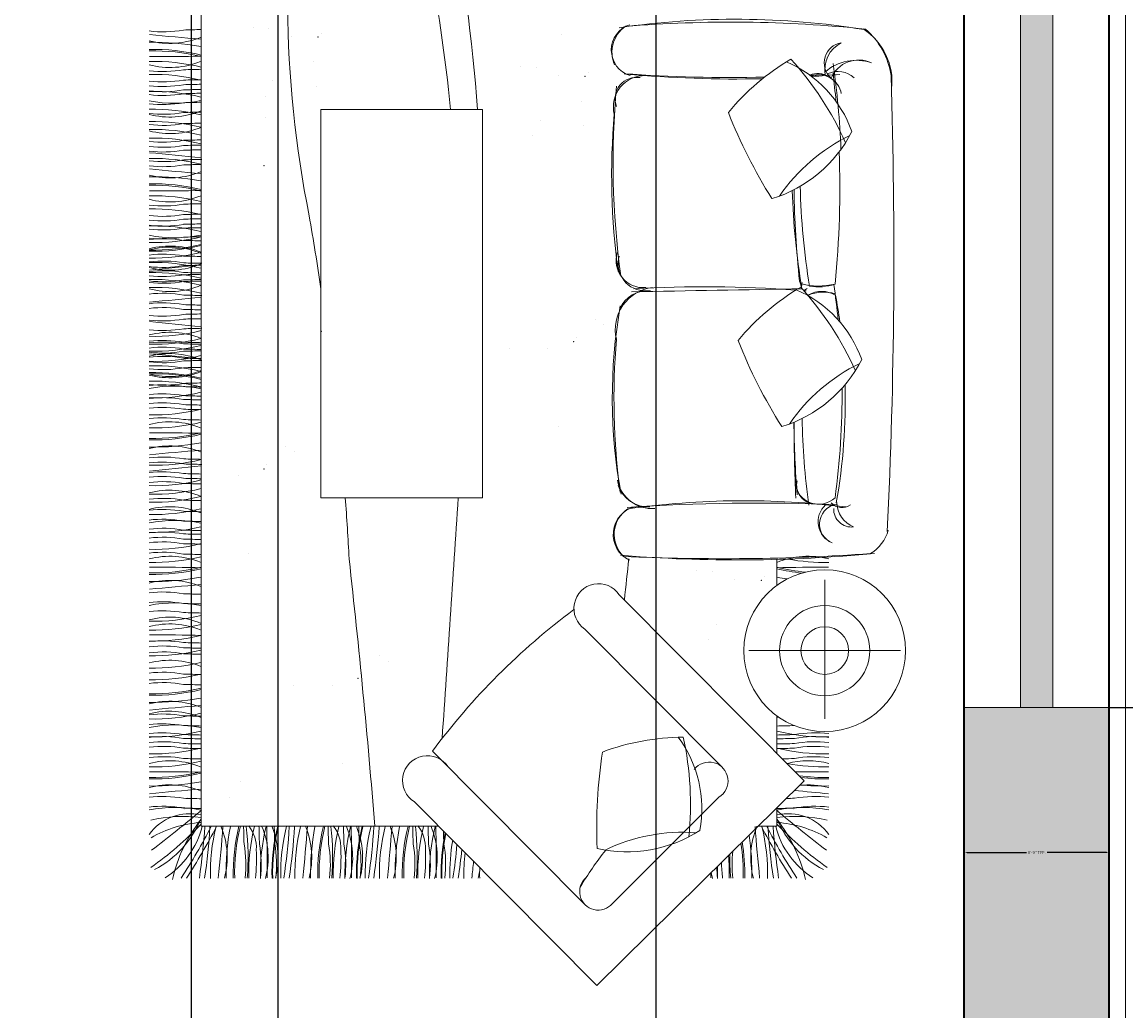
# Model space of a CAD drawing. Units: inches. Extents: x 311 to 815, y -527 to 136.
# Tile 11 of 21: x 655 to 723, y -464 to -403. Entities that reach past the tile are written whole.
import ezdxf

# ---------------------------------------------------------------- set-up
doc = ezdxf.new("R2010")
doc.units = ezdxf.units.IN
doc.header["$MEASUREMENT"] = 0
for name, color, linetype, lineweight in [('A-ANNO-DIMS', 1, 'Continuous', 18), ('A-FLOR-EDGE', 1, 'Continuous', 18), ('A-GLAZ-PATT', 5, 'Continuous', 13), ('A-WALL-PATT', 242, 'Continuous', 13), ('wall', 1, 'Continuous', 35), ('win', 5, 'Continuous', 18)]:
    doc.layers.add(name, color=color, linetype=linetype, lineweight=lineweight)
doc.layers.add('furniture', color=50, linetype='Continuous', lineweight=13, transparency=0.8)
doc.styles.get("Standard").update_dxf_attribs({"font": 'arial.ttf'})
doc.dimstyles.get("Standard").update_dxf_attribs({"dimtxt": 0.18, "dimasz": 0.18, "dimexe": 0.18, "dimexo": 0.0625, "dimgap": 0.09, "dimtad": 0, "dimtih": 1, "dimtoh": 1, "dimdec": 1, "dimzin": 0, "dimdsep": 46, "dimlunit": 4, "dimtxsty": 'Standard', "dimcen": 0.09, "dimadec": 0, "dimazin": 0, "dimtfac": 1, "dimtdec": 1, "dimtofl": 0, "dimtmove": 0, "dimatfit": 3, "dimfxl": 1, "dimtolj": 1, "dimtzin": 0, "dimarcsym": 0})

# ---------------------------------------------------------------- blocks, each defined once
blk = doc.blocks.new('WIN-60IN')
for p, q in [((9, 60), (0, 60)), ((3.5, 0), (3.5, 60)), ((5.5, 0), (5.5, 60)), ((9, 0), (0, 0))]:
    blk.add_line(p, q)
blk = doc.blocks.new('*D10')
at = {"layer": 'A-ANNO-DIMS', "color": 0, "lineweight": -2, "transparency": 16777216}
for p, q in [((722.385, -385.128), (731.503, -385.128)), ((731.323, -385.308), (731.323, -414.945)), ((731.323, -444.948), (731.323, -415.311)), ((722.385, -445.128), (731.503, -445.128))]:
    blk.add_line(p, q, dxfattribs=at)
at = {"layer": 'A-ANNO-DIMS', "color": 0, "transparency": 16777216}
for points in [[(731.293, -385.308), (731.353, -385.308), (731.323, -385.128)], [(731.293, -444.948), (731.353, -444.948), (731.323, -445.128)]]:
    blk.add_solid(points, dxfattribs=at)
at = {"layer": 'Defpoints', "color": 0, "transparency": 16777216}
for p in [(722.323, -385.128), (731.323, -385.128), (722.323, -445.128)]:
    blk.add_point(p, dxfattribs=at)
at = {"layer": 'A-ANNO-DIMS', "color": 0, "transparency": 16777216, "insert": (731.323, -415.128), "char_height": 0.18, "attachment_point": 5}
blk.add_mtext('\\A1;WINDOW 5\'-0" TYP.', dxfattribs=at)
blk = doc.blocks.new('*D11')
at = {"layer": 'A-ANNO-DIMS', "color": 0, "lineweight": -2, "transparency": 16777216}
for p, q in [((713.323, -445.19), (713.323, -454.308)), ((722.323, -445.19), (722.323, -454.308)), ((713.503, -454.128), (717.184, -454.128)), ((722.143, -454.128), (718.461, -454.128))]:
    blk.add_line(p, q, dxfattribs=at)
at = {"layer": 'A-ANNO-DIMS', "color": 0, "transparency": 16777216}
for points in [[(713.503, -454.098), (713.503, -454.158), (713.323, -454.128)], [(722.143, -454.098), (722.143, -454.158), (722.323, -454.128)]]:
    blk.add_solid(points, dxfattribs=at)
at = {"layer": 'Defpoints', "color": 0, "transparency": 16777216}
for p in [(713.323, -445.128), (722.323, -445.128), (722.323, -454.128)]:
    blk.add_point(p, dxfattribs=at)
at = {"layer": 'A-ANNO-DIMS', "color": 0, "transparency": 16777216, "insert": (717.823, -454.128), "char_height": 0.18, "attachment_point": 5}
blk.add_mtext('\\A1;0\'-9" TYP.', dxfattribs=at)
blk = doc.blocks.new('*D30')
at = {"layer": 'A-ANNO-DIMS', "color": 0, "lineweight": -2, "transparency": 16777216}
for p, q in [((722.385, -445.128), (754.853, -445.128)), ((754.673, -445.308), (754.673, -463.446)), ((754.673, -481.948), (754.673, -463.81)), ((722.385, -482.128), (754.853, -482.128))]:
    blk.add_line(p, q, dxfattribs=at)
at = {"layer": 'A-ANNO-DIMS', "color": 0, "transparency": 16777216}
for points in [[(754.643, -445.308), (754.703, -445.308), (754.673, -445.128)], [(754.643, -481.948), (754.703, -481.948), (754.673, -482.128)]]:
    blk.add_solid(points, dxfattribs=at)
at = {"layer": 'Defpoints', "color": 0, "transparency": 16777216}
for p in [(722.323, -445.128), (754.673, -445.128), (722.323, -482.128)]:
    blk.add_point(p, dxfattribs=at)
at = {"layer": 'A-ANNO-DIMS', "color": 0, "transparency": 16777216, "insert": (754.673, -463.628), "char_height": 0.18, "attachment_point": 5}
blk.add_mtext('\\A1;3\'-1"', dxfattribs=at)
blk = doc.blocks.new('*D31')
at = {"layer": 'A-ANNO-DIMS', "color": 0, "lineweight": -2, "transparency": 16777216}
for p, q in [((670.696, -191.608), (670.696, -526.658)), ((694.164, -191.608), (694.164, -526.658)), ((670.876, -526.478), (681.83, -526.478)), ((693.984, -526.478), (683.03, -526.478))]:
    blk.add_line(p, q, dxfattribs=at)
at = {"layer": 'A-ANNO-DIMS', "color": 0, "transparency": 16777216}
for points in [[(670.876, -526.448), (670.876, -526.508), (670.696, -526.478)], [(693.984, -526.448), (693.984, -526.508), (694.164, -526.478)]]:
    blk.add_solid(points, dxfattribs=at)
at = {"layer": 'Defpoints', "color": 0, "transparency": 16777216}
for p in [(670.696, -191.545), (694.164, -191.545), (694.164, -526.478)]:
    blk.add_point(p, dxfattribs=at)
at = {"layer": 'A-ANNO-DIMS', "color": 0, "transparency": 16777216, "insert": (682.43, -526.478), "char_height": 0.18, "attachment_point": 5}
blk.add_mtext('\\A1;1\'-11 1/2"', dxfattribs=at)
blk = doc.blocks.new('*D37')
at = {"layer": 'A-ANNO-DIMS', "color": 0, "lineweight": -2, "transparency": 16777216}
for p, q in [((633.323, -348.19), (633.323, -526.658)), ((665.323, -348.19), (665.323, -526.658)), ((633.503, -526.478), (648.992, -526.478)), ((665.143, -526.478), (649.654, -526.478))]:
    blk.add_line(p, q, dxfattribs=at)
at = {"layer": 'A-ANNO-DIMS', "color": 0, "transparency": 16777216}
for points in [[(633.503, -526.448), (633.503, -526.508), (633.323, -526.478)], [(665.143, -526.448), (665.143, -526.508), (665.323, -526.478)]]:
    blk.add_solid(points, dxfattribs=at)
at = {"layer": 'Defpoints', "color": 0, "transparency": 16777216}
for p in [(633.323, -348.128), (665.323, -348.128), (665.323, -526.478)]:
    blk.add_point(p, dxfattribs=at)
at = {"layer": 'A-ANNO-DIMS', "color": 0, "transparency": 16777216, "insert": (649.323, -526.478), "char_height": 0.18, "attachment_point": 5}
blk.add_mtext('\\A1;2\'-8"', dxfattribs=at)

msp = doc.modelspace()

# ---------------------------------------------------------------- hatches: boundary and pattern name
at = {"layer": 'A-GLAZ-PATT'}
h = msp.add_hatch(color=256, dxfattribs=at)
h.dxf.hatch_style = 1
h.paths.add_polyline_path([(415.823, -202.128), (413.823, -202.128), (413.823, -262.128), (415.823, -262.128)])
h.paths.add_polyline_path([(415.823, -390.84), (413.823, -390.84), (413.823, -450.84), (415.823, -450.84)])
h.paths.add_polyline_path([(415.823, -311.568), (413.823, -311.568), (413.823, -335.568), (415.823, -335.568)])
h.paths.add_polyline_path([(509.323, -476.628), (449.323, -476.628), (449.323, -478.628), (509.323, -478.628)])
h.paths.add_polyline_path([(606.823, -476.628), (582.823, -476.628), (582.823, -478.628), (606.823, -478.628)])
h.paths.add_polyline_path([(678.823, -476.628), (654.823, -476.628), (654.823, -478.628), (678.823, -478.628)])
h.paths.add_polyline_path([(718.823, -385.128), (716.823, -385.128), (716.823, -445.128), (718.823, -445.128)])
h.paths.add_polyline_path([(718.823, -262.628), (716.823, -262.628), (716.823, -322.628), (718.823, -322.628)])
h.paths.add_polyline_path([(718.823, -140.128), (716.823, -140.128), (716.823, -200.128), (718.823, -200.128)])
h.paths.add_polyline_path([(718.823, -18.128), (716.823, -18.128), (716.823, -42.128), (718.823, -42.128)])
h.paths.add_polyline_path([(686.823, 18.372), (626.823, 18.372), (626.823, 16.372), (686.823, 16.372)])
h.paths.add_polyline_path([(581.823, 18.372), (557.823, 18.372), (557.823, 16.372), (581.823, 16.372)])
h.paths.add_polyline_path([(509.323, 18.372), (449.323, 18.372), (449.323, 16.372), (509.323, 16.372)])
at = {"layer": 'A-WALL-PATT'}
h = msp.add_hatch(color=256, dxfattribs=at)
h.dxf.hatch_style = 1
h.paths.add_polyline_path([(557.823, 21.872), (509.323, 21.872), (509.323, 12.872), (539.323, 12.872), (539.323, -112.128), (548.323, -112.128), (548.323, -58.628), (557.823, -58.628), (557.823, -49.628), (548.323, -49.628), (548.323, 12.872), (557.823, 12.872)])
h.paths.add_polyline_path([(449.323, 21.872), (410.323, 21.872), (410.323, -15.128), (419.323, -15.128), (419.323, 12.872), (449.323, 12.872)])
h.paths.add_polyline_path([(626.823, 21.872), (581.823, 21.872), (581.823, 12.872), (591.323, 12.872), (591.323, -49.628), (581.823, -49.628), (581.823, -58.628), (591.323, -58.628), (591.323, -112.128), (600.323, -112.128), (600.323, 12.872), (626.823, 12.872)])
h.paths.add_polyline_path([(722.323, 21.872), (686.823, 21.872), (686.823, 12.872), (713.323, 12.872), (713.323, -18.128), (722.323, -18.128)])
h.paths.add_polyline_path([(722.323, -42.128), (713.323, -42.128), (713.323, -73.128), (722.323, -73.128)])
h.paths.add_polyline_path([(501.323, -103.128), (419.323, -103.128), (419.323, -75.128), (410.323, -75.128), (410.323, -126.628), (419.323, -126.628), (419.323, -112.128), (492.323, -112.128), (492.323, -143.128), (501.323, -143.128)])
h.paths.add_polyline_path([(548.323, -165.128), (419.323, -165.128), (419.323, -150.628), (410.323, -150.628), (410.323, -202.128), (419.323, -202.128), (419.323, -174.128), (548.323, -174.128)])
h.paths.add_polyline_path([(722.323, -103.128), (636.323, -103.128), (636.323, -112.128), (713.323, -112.128), (713.323, -140.128), (722.323, -140.128)])
h.paths.add_polyline_path([(548.323, -210.128), (539.323, -210.128), (539.323, -290.128), (419.323, -290.128), (419.323, -262.128), (410.323, -262.128), (410.323, -311.568), (419.323, -311.568), (419.323, -299.128), (469.323, -299.128), (469.323, -348.128), (443.323, -348.128), (443.323, -357.128), (478.323, -357.128), (478.323, -299.128), (548.323, -299.128)])
h.paths.add_polyline_path([(722.323, -200.128), (713.323, -200.128), (713.323, -228.128), (609.323, -228.128), (609.323, -237.128), (713.323, -237.128), (713.323, -262.628), (722.323, -262.628)])
h.paths.add_polyline_path([(722.323, -322.628), (713.323, -322.628), (713.323, -348.128), (633.323, -348.128), (633.323, -357.128), (713.323, -357.128), (713.323, -385.128), (722.323, -385.128)])
h.paths.add_polyline_path([(419.323, -335.568), (410.323, -335.568), (410.323, -390.84), (419.323, -390.84)])
h.paths.add_polyline_path([(419.323, -450.84), (410.323, -450.84), (410.323, -482.128), (449.323, -482.128), (449.323, -473.128), (419.323, -473.128)])
h.paths.add_polyline_path([(582.823, -473.128), (548.323, -473.128), (548.323, -348.128), (539.323, -348.128), (539.323, -473.128), (509.323, -473.128), (509.323, -482.128), (582.823, -482.128)])
h.paths.add_polyline_path([(722.323, -445.128), (713.323, -445.128), (713.323, -473.128), (678.823, -473.128), (678.823, -482.128), (722.323, -482.128)])

# ---------------------------------------------------------------- linework, layer by layer
at = {"layer": 'A-FLOR-EDGE'}
msp.add_line((723.323, -483.128), (723.323, 22.872), dxfattribs=at)
at = {"layer": 'furniture'}
for p, q in [((665.936, -452.501), (665.936, -388.632)), ((665.936, -398.727), (665.936, -452.501)), ((669.173, -402.89), (669.173, -402.89)), ((670.143, -402.965), (670.143, -402.965)), ((671.534, -403.459), (671.534, -403.459)), ((673.409, -403.275), (673.409, -403.275)), ((688.316, -403.329), (688.316, -403.329)), ((672.946, -405.051), (672.946, -405.051)), ((685.767, -405.34), (685.767, -405.34)), ((686.738, -405.415), (686.738, -405.415)), ((690.003, -405.725), (690.003, -405.725)), ((670.397, -406.214), (670.397, -406.214)), ((688.129, -405.909), (688.129, -405.909)), ((673.075, -406.567), (673.075, -406.567)), ((669.935, -407.168), (669.935, -407.168)), ((689.541, -407.501), (689.541, -407.501)), ((673.371, -408), (683.413, -408)), ((673.371, -432.102), (673.371, -408)), ((683.413, -408), (683.413, -432.102)), ((669.912, -408.488), (669.912, -408.488)), ((686.991, -408.665), (686.991, -408.665)), ((689.67, -409.017), (689.67, -409.017)), ((686.53, -409.618), (686.53, -409.618)), ((664.928, -416.035), (664.928, -416.035)), ((664.928, -416.106), (664.928, -416.106)), ((664.928, -418.285), (664.928, -418.285)), ((690.421, -421.011), (690.421, -421.011)), ((690.421, -421.011), (690.421, -421.011)), ((690.946, -421.359), (690.946, -421.359)), ((690.946, -421.359), (690.946, -421.359)), ((689.22, -422.136), (689.22, -422.136)), ((664.928, -422.848), (664.928, -422.848)), ((687.469, -422.829), (687.469, -422.829)), ((685.087, -422.864), (685.087, -422.864)), ((664.928, -425.027), (664.928, -425.027)), ((664.928, -425.098), (664.928, -425.098)), ((688.108, -427.669), (688.108, -427.669)), ((671.187, -428.913), (671.187, -428.913)), ((671.187, -428.913), (671.187, -428.913)), ((671.712, -429.261), (671.712, -429.261)), ((671.712, -429.261), (671.712, -429.261)), ((669.986, -430.038), (669.986, -430.038)), ((665.853, -430.766), (665.853, -430.766)), ((668.235, -430.73), (668.235, -430.73)), ((683.413, -432.102), (673.371, -432.102)), ((668.874, -435.571), (668.874, -435.571)), ((701.687, -435.93), (701.687, -437.547)), ((696.705, -436.628), (696.705, -436.628)), ((697.675, -436.702), (697.675, -436.702)), ((699.066, -437.197), (699.066, -437.197)), ((700.941, -437.012), (700.941, -437.012)), ((704.658, -441.595), (704.658, -437.2)), ((703.381, -449.674), (691.898, -438.125)), ((697.929, -439.952), (697.929, -439.952)), ((698.312, -448.858), (689.768, -440.255)), ((697.467, -440.905), (697.467, -440.905)), ((677.033, -441.918), (677.033, -441.918)), ((677.033, -441.918), (677.033, -441.918)), ((704.658, -441.595), (699.955, -441.595)), ((704.658, -441.595), (704.658, -445.828)), ((704.658, -441.595), (709.36, -441.595)), ((677.558, -442.266), (677.558, -442.266)), ((677.558, -442.266), (677.558, -442.266)), ((675.832, -443.043), (675.832, -443.043)), ((671.699, -443.771), (671.699, -443.771)), ((674.081, -443.735), (674.081, -443.735)), ((701.687, -445.643), (701.687, -447.971)), ((680.299, -447.842), (689.78, -457.369)), ((674.72, -448.576), (674.72, -448.576)), ((668.364, -449.733), (668.364, -449.733)), ((703.381, -449.674), (690.515, -462.379)), ((665.118, -450.713), (665.118, -450.713)), ((665.118, -450.713), (665.118, -450.713)), ((665.118, -450.713), (665.118, -450.713)), ((667.679, -450.695), (667.679, -450.695)), ((698.077, -450.697), (691.477, -457.296)), ((698.077, -450.697), (697.019, -451.755)), ((702.505, -450.713), (702.505, -450.713)), ((702.505, -450.713), (702.505, -450.713)), ((702.505, -450.713), (702.505, -450.713)), ((664.928, -451.486), (664.928, -451.486)), ((664.928, -451.486), (664.928, -451.486)), ((664.928, -451.486), (664.928, -451.486)), ((690.515, -462.379), (679.179, -450.979)), ((701.687, -451.347), (701.687, -452.501)), ((702.695, -451.486), (702.695, -451.486)), ((702.695, -451.486), (702.695, -451.486)), ((702.695, -451.486), (702.695, -451.486)), ((680.693, -452.501), (665.936, -452.501)), ((701.687, -452.501), (700.518, -452.501)), ((695.158, -453.615), (691.477, -457.296)), ((670.763, -454.219), (670.763, -454.219)), ((676.009, -454.219), (676.009, -454.219)), ((681.262, -454.219), (681.262, -454.219)), ((670.738, -454.523), (670.738, -454.523)), ((675.984, -454.523), (675.984, -454.523)), ((681.237, -454.523), (681.237, -454.523))]:
    msp.add_line(p, q, dxfattribs=at)
for radius in [5.021, 2.803, 1.481]:
    msp.add_circle((704.658, -441.595), radius, dxfattribs=at)
for centre, radius, start, end in [((741.561, -400.92), 70.258, 169.92753, 191.22459), ((587.613, -416.937), 94.235, 5.44209, 17.47988), ((537.566, -419.76), 146.015, 4.61959, 9.75131), ((693.064, -404.316), 1.657, 107.71573, 252.84284), ((693.448, -404.459), 2, 126.0678, 202.6723), ((699.135, -452.295), 49.897, 80.80787, 98.3514), ((698.81, -483.677), 81.099, 84.0627, 94.62528), ((663.574, -395.915), 7.265, 263.11705, 280.06509), ((664.003, -398.882), 5.018, 255.13868, 292.69016), ((677.166, -261.215), 142.863, 264.19829, 265.48538), ((667.404, -484.064), 81.037, 91.02248, 91.81091), ((704.912, -406.292), 3.923, 353.87925, 57.10928), ((704.032, -406.62), 4.8, 8.65495, 48.71038), ((662.987, -420.078), 16.251, 79.59608, 90.98046), ((663.005, -416.508), 12.239, 76.14265, 91.36693), ((705.887, -405.1), 1.263, 99.29162, 227.62886), ((706.582, -405.556), 1.925, 117.84326, 189.86837), ((663.004, -417.253), 12.239, 76.14265, 91.36693), ((663.005, -416.599), 12.239, 76.14265, 91.36693), ((664, -400.377), 5.018, 255.13868, 292.69016), ((663.458, -299.941), 104.775, 269.60659, 271.37204), ((709.882, -417.405), 14.512, 120.30685, 140.5663), ((699.365, -411.841), 7.4, 19.45006, 66.76991), ((688.059, -418.059), 19.597, 24.08153, 42.27682), ((706.614, -407.901), 2.952, 71.24727, 131.13483), ((706.769, -406.797), 1.868, 64.87152, 156.7247), ((663.581, -398.382), 7.265, 263.11705, 280.06509), ((667.411, -486.531), 81.037, 91.02248, 91.81091), ((705.48, -407.13), 1.491, 47.72028, 114.44608), ((655.363, -412.415), 50.34, 2.2017, 8.30671), ((663.579, -399.024), 7.265, 263.11705, 280.06509), ((663.002, -418.063), 12.239, 76.14265, 91.36693), ((667.41, -487.174), 81.037, 91.02248, 91.81091), ((693.462, -407.828), 1.929, 87.65794, 194.09744), ((692.978, -407.341), 1.336, 80.26169, 201.01149), ((698.759, -316.368), 89.651, 265.80271, 271.38032), ((699.078, -332.35), 73.76, 264.74224, 271.33354), ((704.211, -407.043), 1.273, 57.73663, 112.23873), ((698.759, -316.368), 89.651, 273.19084, 273.78915), ((704.289, -407.275), 1.421, 10.62162, 109.19299), ((699.078, -332.35), 73.76, 273.71005, 275.06529), ((644.917, -412.878), 60.679, 5.08707, 6.74912), ((349.903, -417.097), 359.048, 357.2697, 1.7875), ((663.577, -399.868), 7.265, 263.11705, 280.06509), ((663.578, -399.633), 7.265, 263.11705, 280.06509), ((662.999, -419.116), 12.239, 76.14265, 91.36693), ((663.578, -399.312), 7.265, 263.11705, 280.06509), ((667.407, -488.017), 81.037, 91.02248, 91.81091), ((667.408, -487.782), 81.037, 91.02248, 91.81091), ((667.409, -487.461), 81.037, 91.02248, 91.81091), ((743.964, -411.292), 52.447, 174.82447, 187.71479), ((663.575, -400.428), 7.265, 263.11705, 280.06509), ((664.295, -399.481), 8.138, 258.75453, 281.58879), ((667.406, -488.577), 81.037, 91.02248, 91.81091), ((663.574, -401.035), 7.265, 263.11705, 280.06509), ((662.996, -420.226), 12.239, 76.14265, 91.36693), ((663.992, -403.454), 5.018, 255.13868, 292.69016), ((667.404, -489.184), 81.037, 91.02248, 91.81091), ((735.84, -412.109), 44.413, 175.07811, 187.69498), ((727.594, -396.89), 31.049, 201.33709, 212.41765), ((662.997, -420.987), 12.239, 76.14265, 91.36693), ((663.584, -401.724), 7.265, 263.11705, 280.06509), ((664.005, -404.48), 5.018, 255.13868, 292.69016), ((667.415, -489.874), 81.037, 91.02248, 91.81091), ((663.007, -422.016), 12.239, 76.14265, 91.36693), ((663.008, -421.481), 12.239, 76.14265, 91.36693), ((698.958, -405.605), 8.293, 287.0126, 332.9429), ((711.121, -419.709), 11.224, 115.90051, 145.65125), ((663.584, -403.084), 7.265, 263.11705, 280.06509), ((663.585, -402.763), 7.265, 263.11705, 280.06509), ((667.405, -491.527), 81.037, 91.02248, 91.81091), ((667.415, -491.233), 81.037, 91.02248, 91.81091), ((667.415, -490.912), 81.037, 91.02248, 91.81091), ((663.574, -403.377), 7.265, 263.11705, 280.06509), ((663.01, -423.28), 12.239, 76.14265, 91.36693), ((663.592, -403.975), 7.265, 263.11705, 280.06509), ((637.626, -681.199), 271.677, 84.01654, 84.69917), ((667.422, -492.124), 81.037, 91.02248, 91.81091), ((644.917, -412.878), 60.679, 354.36393, 2.12187), ((664.003, -407.228), 5.018, 255.13868, 292.69016), ((663.587, -404.288), 7.265, 263.11705, 280.06509), ((677.166, -269.561), 142.863, 264.19829, 265.48538), ((667.418, -492.437), 81.037, 91.02248, 91.81091), ((662.987, -428.423), 16.251, 79.59608, 90.98046), ((663.005, -424.854), 12.239, 76.14265, 91.36693), ((663.005, -424.945), 12.239, 76.14265, 91.36693), ((663.458, -308.286), 104.775, 269.60659, 271.37204), ((747.074, -411.756), 44.447, 181.64583, 189.52678), ((758.639, -412.494), 55.884, 180.49489, 186.32914), ((744.759, -412.035), 41.624, 181.00607, 189.60009), ((663.581, -406.728), 7.265, 263.11705, 280.06509), ((663.004, -425.599), 12.239, 76.14265, 91.36693), ((664, -408.723), 5.018, 255.13868, 292.69016), ((667.411, -494.877), 81.037, 91.02248, 91.81091), ((663.579, -407.37), 7.265, 263.11705, 280.06509), ((663.002, -426.409), 12.239, 76.14265, 91.36693), ((667.41, -495.519), 81.037, 91.02248, 91.81091), ((538.237, -438.403), 136.502, 8.11901, 10.04424), ((663.578, -407.978), 7.265, 263.11705, 280.06509), ((662.999, -427.461), 12.239, 76.14265, 91.36693), ((663.578, -407.657), 7.265, 263.11705, 280.06509), ((667.408, -496.127), 81.037, 91.02248, 91.81091), ((667.409, -495.807), 81.037, 91.02248, 91.81091), ((663.575, -408.774), 7.265, 263.11705, 280.06509), ((663.577, -408.214), 7.265, 263.11705, 280.06509), ((664.295, -407.827), 8.138, 258.75453, 281.58879), ((663.007, -404.029), 12.239, 268.63307, 283.85735), ((667.406, -496.923), 81.037, 91.02248, 91.81091), ((667.407, -496.363), 81.037, 91.02248, 91.81091), ((663.585, -423.282), 7.265, 79.93491, 96.88295), ((663.008, -404.493), 12.239, 268.63307, 283.85735), ((663.008, -404.564), 12.239, 268.63307, 283.85735), ((664.005, -421.494), 5.018, 67.30984, 104.86132), ((664.005, -421.565), 5.018, 67.30984, 104.86132), ((667.415, -335.132), 81.037, 268.18909, 268.97752), ((662.997, -404.987), 12.239, 268.63307, 283.85735), ((663.584, -424.25), 7.265, 79.93491, 96.88295), ((667.415, -336.101), 81.037, 268.18909, 268.97752), ((693.39, -417.372), 1.691, 162.93165, 275.10915), ((693.511, -417.581), 1.676, 163.4437, 271.82282), ((663.574, -410.542), 7.265, 263.11705, 280.06509), ((662.996, -429.733), 12.239, 76.14265, 91.36693), ((663.574, -425.274), 7.265, 79.93491, 96.88295), ((663.992, -412.961), 5.018, 255.13868, 292.69016), ((663.592, -424.676), 7.265, 79.93491, 96.88295), ((637.626, -147.452), 271.677, 275.30083, 275.98346), ((667.404, -498.691), 81.037, 91.02248, 91.81091), ((667.422, -336.527), 81.037, 268.18909, 268.97752), ((662.997, -430.791), 12.239, 76.14265, 91.36693), ((663.584, -411.43), 7.265, 263.11705, 280.06509), ((663.585, -411.109), 7.265, 263.11705, 280.06509), ((663.584, -411.529), 7.265, 263.11705, 280.06509), ((663.007, -430.361), 12.239, 76.14265, 91.36693), ((667.405, -337.124), 81.037, 268.18909, 268.97752), ((667.415, -499.579), 81.037, 91.02248, 91.81091), ((667.415, -499.678), 81.037, 91.02248, 91.81091), ((667.415, -499.258), 81.037, 91.02248, 91.81091), ((686.135, -423.99), 17.781, 15.96247, 17.46375), ((789.397, -427.959), 86.636, 173.88721, 174.12153), ((663.008, -431.286), 12.239, 76.14265, 91.36693), ((664.005, -414.285), 5.018, 255.13868, 292.69016), ((663.592, -426.673), 7.265, 79.93491, 96.88295), ((694.273, -421.657), 2.617, 96.58671, 193.45107), ((693.668, -421.168), 1.911, 84.92344, 155.63742), ((-15074.083, 884137.718), 884697.543, 271.021158169, 271.0218453), ((697.245, -496.583), 77.577, 85.84252, 93.2873), ((710.49, -431.56), 14.512, 120.30685, 140.5663), ((699.974, -425.996), 7.4, 19.45006, 66.76991), ((704.285, -414.819), 4.145, 254.04794, 284.20605), ((688.668, -432.214), 19.597, 24.08153, 42.27682), ((697.245, -496.583), 77.577, 85.36553, 85.4784), ((704.071, -420.036), 1.053, 119.13127, 132.01414), ((704.594, -421.806), 2.471, 73.31083, 112.61636), ((704.471, -420.974), 1.679, 59.83188, 119.46797), ((704.219, -415.607), 3.407, 261.53624, 288.34934), ((659.2, -425.759), 46.534, 5.77953, 8.52202), ((663.574, -427.271), 7.265, 79.93491, 96.88295), ((637.626, -149.449), 271.677, 275.30083, 275.98346), ((667.405, -339.121), 81.037, 268.18909, 268.97752), ((667.422, -338.524), 81.037, 268.18909, 268.97752), ((754.132, -425.971), 50.898, 172.72451, 172.77255), ((669.76, -426.096), 36.171, 7.80299, 10.45572), ((663.584, -427.564), 7.265, 79.93491, 96.88295), ((663.584, -413.569), 7.265, 263.11705, 280.06509), ((667.415, -339.415), 81.037, 268.18909, 268.97752), ((667.415, -501.718), 81.037, 91.02248, 91.81091), ((724.548, -425.909), 33.08, 170.0543, 190.4167), ((663.574, -413.863), 7.265, 263.11705, 280.06509), ((637.626, -691.684), 271.677, 84.01654, 84.69917), ((667.405, -502.012), 81.037, 91.02248, 91.81091), ((663.008, -409.848), 12.239, 268.63307, 283.85735), ((664.005, -426.849), 5.018, 67.30984, 104.86132), ((663.592, -414.46), 7.265, 263.11705, 280.06509), ((667.422, -502.609), 81.037, 91.02248, 91.81091), ((662.997, -410.342), 12.239, 268.63307, 283.85735), ((663.584, -429.703), 7.265, 79.93491, 96.88295), ((663.584, -429.604), 7.265, 79.93491, 96.88295), ((663.585, -430.024), 7.265, 79.93491, 96.88295), ((663.007, -410.772), 12.239, 268.63307, 283.85735), ((667.415, -341.455), 81.037, 268.18909, 268.97752), ((667.415, -341.554), 81.037, 268.18909, 268.97752), ((735.74, -425.956), 44.167, 175.20718, 187.55097), ((728.203, -411.045), 31.049, 201.33709, 212.41765), ((663.574, -430.591), 7.265, 79.93491, 96.88295), ((663.574, -415.86), 7.265, 263.11705, 280.06509), ((662.996, -411.4), 12.239, 268.63307, 283.85735), ((663.992, -428.172), 5.018, 67.30984, 104.86132), ((637.626, -693.681), 271.677, 84.01654, 84.69917), ((667.404, -342.442), 81.037, 268.18909, 268.97752), ((667.405, -504.009), 81.037, 91.02248, 91.81091), ((667.415, -341.875), 81.037, 268.18909, 268.97752), ((699.566, -419.76), 8.293, 287.0126, 332.9429), ((662.997, -436.146), 12.239, 76.14265, 91.36693), ((663.584, -416.883), 7.265, 263.11705, 280.06509), ((664.005, -419.568), 5.018, 255.13868, 292.69016), ((663.592, -416.457), 7.265, 263.11705, 280.06509), ((667.415, -505.033), 81.037, 91.02248, 91.81091), ((667.422, -504.606), 81.037, 91.02248, 91.81091), ((711.73, -433.863), 11.224, 115.90051, 145.65125), ((663.007, -437.104), 12.239, 76.14265, 91.36693), ((663.008, -436.569), 12.239, 76.14265, 91.36693), ((663.008, -436.64), 12.239, 76.14265, 91.36693), ((664.005, -419.639), 5.018, 255.13868, 292.69016), ((663.575, -432.359), 7.265, 79.93491, 96.88295), ((664.295, -433.306), 8.138, 78.41121, 101.24547), ((662.999, -413.672), 12.239, 268.63307, 283.85735), ((663.585, -417.852), 7.265, 263.11705, 280.06509), ((667.406, -344.21), 81.037, 268.18909, 268.97752), ((667.415, -506.001), 81.037, 91.02248, 91.81091), ((659.2, -425.759), 46.534, 352.15508, 0.55852), ((669.76, -426.096), 36.171, 349.94664, 1.59031), ((663.577, -432.919), 7.265, 79.93491, 96.88295), ((663.578, -433.155), 7.265, 79.93491, 96.88295), ((663.578, -433.476), 7.265, 79.93491, 96.88295), ((667.407, -344.77), 81.037, 268.18909, 268.97752), ((667.408, -345.006), 81.037, 268.18909, 268.97752), ((663.579, -433.763), 7.265, 79.93491, 96.88295), ((663.002, -414.725), 12.239, 268.63307, 283.85735), ((667.409, -345.327), 81.037, 268.18909, 268.97752), ((667.41, -345.614), 81.037, 268.18909, 268.97752), ((663.581, -434.405), 7.265, 79.93491, 96.88295), ((663.004, -415.534), 12.239, 268.63307, 283.85735), ((664, -432.41), 5.018, 67.30984, 104.86132), ((667.411, -346.256), 81.037, 268.18909, 268.97752), ((772.401, -426.514), 69.666, 180.7456, 184.45597), ((789.397, -427.959), 86.636, 179.63856, 182.76525), ((754.132, -425.971), 50.898, 181.37312, 187.44721), ((663.005, -416.188), 12.239, 268.63307, 283.85735), ((663.005, -416.279), 12.239, 268.63307, 283.85735), ((663.458, -532.847), 104.775, 88.62796, 90.39341), ((662.987, -412.71), 16.251, 269.01954, 280.40392), ((664.003, -433.905), 5.018, 67.30984, 104.86132), ((663.587, -436.845), 7.265, 79.93491, 96.88295), ((677.166, -571.573), 142.863, 94.51462, 95.80171), ((667.418, -348.696), 81.037, 268.18909, 268.97752), ((663.01, -417.853), 12.239, 268.63307, 283.85735), ((663.592, -437.158), 7.265, 79.93491, 96.88295), ((637.626, -159.934), 271.677, 275.30083, 275.98346), ((667.422, -349.009), 81.037, 268.18909, 268.97752), ((663.574, -437.756), 7.265, 79.93491, 96.88295), ((663.584, -438.049), 7.265, 79.93491, 96.88295), ((663.007, -419.117), 12.239, 268.63307, 283.85735), ((667.405, -349.607), 81.037, 268.18909, 268.97752), ((667.415, -349.9), 81.037, 268.18909, 268.97752), ((693.923, -430.603), 2.173, 190.97559, 274.97468), ((704.085, -431.313), 1.171, 167.62255, 260.30943), ((663.585, -438.37), 7.265, 79.93491, 96.88295), ((663.008, -419.652), 12.239, 268.63307, 283.85735), ((664.005, -436.653), 5.018, 67.30984, 104.86132), ((667.415, -350.221), 81.037, 268.18909, 268.97752), ((693.721, -430.663), 2.012, 199.82281, 272.49854), ((704.289, -431.031), 1.478, 186.1174, 313.1189), ((662.997, -420.146), 12.239, 268.63307, 283.85735), ((663.584, -439.409), 7.265, 79.93491, 96.88295), ((667.415, -351.26), 81.037, 268.18909, 268.97752), ((546.734, -442.144), 128.547, 2.78771, 4.48071), ((-2183.497, -248.346), 2871.284, 356.03178, 356.330686), ((700.403, -548.527), 116.093, 87.50734, 93.9592), ((699.641, -484.084), 51.795, 82.98362, 97.98903), ((705.734, -431.758), 0.952, 224.39377, 303.58565), ((707.087, -432.358), 1.684, 181.18396, 247.82163), ((663.574, -440.098), 7.265, 79.93491, 96.88295), ((662.996, -420.907), 12.239, 268.63307, 283.85735), ((663.992, -437.679), 5.018, 67.30984, 104.86132), ((667.404, -351.949), 81.037, 268.18909, 268.97752), ((693.303, -434.381), 1.776, 104.63788, 244.30948), ((693.474, -434.379), 1.893, 123.04105, 226.06525), ((705.655, -433.596), 1.413, 132.31343, 247.61024), ((705.597, -433.738), 1.26, 104.78136, 247.59217), ((706.324, -432.812), 1.112, 178.0108, 276.55846), ((663.575, -440.705), 7.265, 79.93491, 96.88295), ((664.295, -441.652), 8.138, 78.41121, 101.24547), ((667.406, -352.556), 81.037, 268.18909, 268.97752), ((663.577, -441.265), 7.265, 79.93491, 96.88295), ((662.999, -422.017), 12.239, 268.63307, 283.85735), ((663.578, -441.501), 7.265, 79.93491, 96.88295), ((667.407, -353.116), 81.037, 268.18909, 268.97752), ((667.408, -353.351), 81.037, 268.18909, 268.97752), ((706.165, -433.422), 2.536, 301.88171, 343.96721), ((663.578, -441.821), 7.265, 79.93491, 96.88295), ((663.579, -442.109), 7.265, 79.93491, 96.88295), ((663.002, -423.07), 12.239, 268.63307, 283.85735), ((667.409, -353.672), 81.037, 268.18909, 268.97752), ((667.41, -353.96), 81.037, 268.18909, 268.97752), ((663.581, -442.751), 7.265, 79.93491, 96.88295), ((663.004, -423.88), 12.239, 268.63307, 283.85735), ((664, -440.756), 5.018, 67.30984, 104.86132), ((667.411, -354.602), 81.037, 268.18909, 268.97752), ((699.186, -345.407), 90.558, 265.43246, 275.43098), ((698.389, -302.976), 132.912, 267.31429, 273.93296), ((703.623, -440.756), 5.018, 75.13868, 112.69016), ((663.005, -424.534), 12.239, 268.63307, 283.85735), ((663.005, -424.625), 12.239, 268.63307, 283.85735), ((663.458, -541.192), 104.775, 88.62796, 90.39341), ((85.648, -501.084), 593.075, 4.698728, 6.310761), ((1281.976, -501.084), 593.075, 173.689239, 173.937357), ((704.166, -541.192), 104.775, 89.60659, 91.37204), ((704.619, -424.534), 12.239, 256.14265, 264.58544), ((704.619, -424.625), 12.239, 256.14265, 263.44666), ((704.62, -423.88), 12.239, 259.37308, 271.36693), ((662.987, -421.055), 16.251, 269.01954, 280.40392), ((664.003, -442.251), 5.018, 67.30984, 104.86132), ((704.637, -421.055), 16.251, 259.59608, 261.86196), ((677.166, -579.918), 142.863, 94.51462, 95.80171), ((690.619, -438.976), 1.536, 33.6335, 236.3665), ((663.574, -445.218), 7.265, 79.93491, 96.88295), ((663.575, -445.825), 7.265, 79.93491, 96.88295), ((667.404, -357.069), 81.037, 268.18909, 268.97752), ((663.577, -446.385), 7.265, 79.93491, 96.88295), ((664.295, -446.772), 8.138, 78.41121, 101.24547), ((667.406, -357.676), 81.037, 268.18909, 268.97752), ((667.407, -358.236), 81.037, 268.18909, 268.97752), ((714.586, -473.31), 42.711, 126.66127, 143.39506), ((663.004, -428.08), 12.239, 268.63307, 283.85735), ((664, -444.956), 5.018, 67.30984, 104.86132), ((663.008, -427.533), 12.239, 268.63307, 283.85735), ((664.005, -444.534), 5.018, 67.30984, 104.86132), ((662.999, -428.766), 12.239, 268.63307, 283.85735), ((663.458, -545.392), 104.775, 88.62796, 90.39341), ((663.578, -448.249), 7.265, 79.93491, 96.88295), ((663.578, -448.57), 7.265, 79.93491, 96.88295), ((667.408, -360.1), 81.037, 268.18909, 268.97752), ((662.997, -429.679), 12.239, 268.63307, 283.85735), ((663.584, -448.942), 7.265, 79.93491, 96.88295), ((667.409, -360.421), 81.037, 268.18909, 268.97752), ((667.415, -360.793), 81.037, 268.18909, 268.97752), ((662.996, -430.44), 12.239, 268.63307, 283.85735), ((663.992, -447.212), 5.018, 67.30984, 104.86132), ((663.579, -450.202), 7.265, 79.93491, 96.88295), ((663.002, -431.164), 12.239, 268.63307, 283.85735), ((667.41, -362.053), 81.037, 268.18909, 268.97752), ((663.581, -450.844), 7.265, 79.93491, 96.88295), ((663.005, -432.037), 12.239, 268.63307, 283.85735), ((663.005, -432.129), 12.239, 268.63307, 283.85735), ((667.411, -362.695), 81.037, 268.18909, 268.97752), ((662.987, -428.559), 16.251, 269.01954, 280.40392), ((664.003, -449.755), 5.018, 67.30984, 104.86132), ((663.992, -450.374), 5.018, 67.30984, 104.86132), ((677.166, -587.422), 142.863, 94.51462, 95.80171), ((663.574, -452.793), 7.265, 79.93491, 96.88295), ((662.996, -433.602), 12.239, 268.63307, 283.85735), ((663.575, -453.4), 7.265, 79.93491, 96.88295), ((667.404, -364.644), 81.037, 268.18909, 268.97752), ((700.219, -364.644), 81.037, 271.02248, 271.06056), ((703.631, -450.374), 5.018, 111.65199, 112.69016), ((663.577, -453.96), 7.265, 79.93491, 96.88295), ((664.295, -454.347), 8.138, 78.41121, 101.24547), ((662.999, -434.712), 12.239, 268.63307, 283.85735), ((667.406, -365.251), 81.037, 268.18909, 268.97752), ((667.407, -365.811), 81.037, 268.18909, 268.97752), ((700.216, -365.811), 81.037, 271.02248, 271.81091), ((700.218, -365.251), 81.037, 271.02248, 271.81091), ((704.625, -434.712), 12.239, 256.14265, 271.36693), ((704.047, -453.96), 7.265, 83.11705, 100.06509), ((663.578, -454.195), 7.265, 79.93491, 96.88295), ((663.578, -454.516), 7.265, 79.93491, 96.88295), ((667.408, -366.046), 81.037, 268.18909, 268.97752), ((667.409, -366.367), 81.037, 268.18909, 268.97752), ((695.953, -461.478), 14.512, 90.30685, 110.5663), ((689.627, -451.402), 7.4, 349.45006, 36.76991), ((676.727, -451.134), 19.597, 354.08153, 12.27682), ((700.215, -366.367), 81.037, 271.02248, 271.81091), ((700.216, -366.046), 81.037, 271.02248, 271.81091), ((704.046, -454.195), 7.265, 83.11705, 100.06509), ((704.045, -454.516), 7.265, 83.11705, 100.06509), ((663.579, -454.804), 7.265, 79.93491, 96.88295), ((663.002, -435.765), 12.239, 268.63307, 283.85735), ((663.581, -455.446), 7.265, 79.93491, 96.88295), ((667.41, -366.655), 81.037, 268.18909, 268.97752), ((679.986, -449.662), 1.544, 33.09238, 238.53066), ((721.55, -452.568), 31.049, 171.33709, 182.41765), ((700.214, -366.655), 81.037, 271.02248, 271.81091), ((704.622, -435.765), 12.239, 256.14265, 271.36693), ((704.043, -455.446), 7.265, 83.11705, 100.06509), ((704.044, -454.804), 7.265, 83.11705, 100.06509), ((663.004, -436.575), 12.239, 268.63307, 283.85735), ((664, -453.451), 5.018, 67.30984, 104.86132), ((667.411, -367.297), 81.037, 268.18909, 268.97752), ((697.482, -449.686), 1.172, 300.48188, 142.32523), ((700.212, -367.297), 81.037, 271.2964, 271.81091), ((703.623, -453.451), 5.018, 75.13868, 104.83406), ((704.62, -436.575), 12.239, 259.25336, 271.36693), ((663.005, -437.229), 12.239, 268.63307, 283.85735), ((663.005, -437.32), 12.239, 268.63307, 283.85735), ((663.458, -553.887), 104.775, 88.62796, 90.39341), ((704.166, -553.887), 104.775, 89.60659, 90.73035), ((704.619, -437.229), 12.239, 262.7707, 271.36693), ((704.619, -437.32), 12.239, 263.2584, 271.36693), ((662.987, -433.75), 16.251, 269.01954, 280.40392), ((664.003, -454.946), 5.018, 67.30984, 104.86132), ((677.166, -592.613), 142.863, 94.51462, 95.80171), ((703.621, -454.946), 5.018, 75.13868, 96.00411), ((704.637, -433.75), 16.251, 264.64881, 270.98046), ((663.574, -457.913), 7.265, 79.93491, 96.88295), ((667.404, -369.764), 81.037, 268.18909, 268.97752), ((700.219, -369.764), 81.037, 271.46162, 271.81091), ((690.457, -592.613), 142.863, 84.19829, 85.05746), ((704.05, -457.913), 7.265, 83.11705, 100.06509), ((663.575, -458.52), 7.265, 79.93491, 96.88295), ((664.295, -459.467), 8.138, 78.41121, 101.24547), ((602.458, -375.386), 99.132, 307.54408, 309.84318), ((667.406, -370.371), 81.037, 268.18909, 268.97752), ((765.166, -375.386), 99.132, 230.15682, 232.45592), ((700.218, -370.371), 81.037, 271.02248, 271.81091), ((703.329, -459.467), 8.138, 78.75453, 101.58879), ((704.048, -458.52), 7.265, 83.11705, 100.06509), ((665.244, -454.843), 3.126, 77.19461, 144.09429), ((664.838, -460.71), 8.827, 82.85092, 103.27854), ((666.483, -459.572), 7.336, 94.27565, 119.86497), ((660.203, -449.686), 6.189, 297.30329, 337.88189), ((673.427, -457.935), 9.516, 141.9231, 167.04771), ((702.38, -454.843), 3.126, 35.90571, 102.80539), ((702.786, -460.71), 8.827, 76.72146, 97.14908), ((707.421, -449.686), 6.189, 202.11811, 242.69671), ((694.196, -457.935), 9.516, 12.95229, 38.0769), ((701.14, -459.572), 7.336, 60.13503, 85.72435), ((650.334, -437.447), 21.587, 305.31527, 316.284), ((660.88, -451.227), 5.282, 302.27123, 346.00651), ((634.552, -436.002), 36.02, 326.82194, 332.73315), ((634.877, -436.01), 36.02, 326.82194, 332.73315), ((631.241, -450.469), 34.984, 351.37714, 356.63558), ((631.566, -450.477), 34.984, 351.37714, 356.63558), ((678.75, -455.439), 12.239, 166.14265, 181.36693), ((524.875, -441.271), 142.863, 354.19829, 355.48538), ((662.542, -454.435), 5.018, 345.13868, 22.69016), ((683.738, -455.451), 16.251, 169.59608, 180.98046), ((680.168, -455.433), 12.239, 166.14265, 181.36693), ((680.259, -455.433), 12.239, 166.14265, 181.36693), ((749.601, -451.026), 81.037, 181.02248, 181.81091), ((652.323, -454.431), 16.533, 355.49364, 6.62982), ((681.133, -455.436), 12.239, 166.14265, 181.36693), ((667.182, -453.832), 2.188, 356.82563, 38.34356), ((750.556, -451.03), 81.037, 181.02248, 181.81091), ((681.857, -455.442), 12.239, 166.14265, 181.36693), ((665.085, -454.445), 5.018, 345.13868, 22.69016), ((565.264, -454.98), 104.775, 359.60659, 1.37204), ((665.7, -454.437), 5.018, 345.13868, 22.69016), ((682.576, -455.434), 12.239, 166.14265, 181.36693), ((682.617, -455.44), 12.239, 166.14265, 181.36693), ((751.504, -451.023), 81.037, 181.02248, 181.81091), ((683.123, -455.429), 12.239, 166.14265, 181.36693), ((636.487, -450.469), 34.984, 351.37714, 356.63558), ((636.813, -450.477), 34.984, 351.37714, 356.63558), ((683.997, -455.439), 12.239, 166.14265, 181.36693), ((530.121, -441.271), 142.863, 354.19829, 355.48538), ((667.789, -454.435), 5.018, 345.13868, 22.69016), ((688.984, -455.451), 16.251, 169.59608, 180.98046), ((685.415, -455.433), 12.239, 166.14265, 181.36693), ((685.506, -455.433), 12.239, 166.14265, 181.36693), ((754.848, -451.026), 81.037, 181.02248, 181.81091), ((657.57, -454.431), 16.533, 355.49364, 6.62982), ((686.379, -455.436), 12.239, 166.14265, 181.36693), ((672.428, -453.832), 2.188, 356.82563, 38.34356), ((755.803, -451.03), 81.037, 181.02248, 181.81091), ((687.104, -455.442), 12.239, 166.14265, 181.36693), ((670.332, -454.445), 5.018, 345.13868, 22.69016), ((570.51, -454.98), 104.775, 359.60659, 1.37204), ((670.947, -454.437), 5.018, 345.13868, 22.69016), ((687.823, -455.434), 12.239, 166.14265, 181.36693), ((687.864, -455.44), 12.239, 166.14265, 181.36693), ((756.751, -451.023), 81.037, 181.02248, 181.81091), ((688.37, -455.429), 12.239, 166.14265, 181.36693), ((641.74, -450.469), 34.984, 351.37714, 356.63558), ((642.065, -450.477), 34.984, 351.37714, 356.63558), ((689.249, -455.439), 12.239, 166.14265, 181.36693), ((535.374, -441.271), 142.863, 354.19829, 355.48538), ((673.041, -454.435), 5.018, 345.13868, 22.69016), ((694.236, -455.451), 16.251, 169.59608, 180.98046), ((690.667, -455.433), 12.239, 166.14265, 181.36693), ((690.758, -455.433), 12.239, 166.14265, 181.36693), ((760.1, -451.026), 81.037, 181.02248, 181.81091), ((662.822, -454.431), 16.533, 355.49364, 6.62982), ((691.632, -455.436), 12.239, 166.14265, 181.36693), ((677.681, -453.832), 2.188, 356.82563, 38.34356), ((761.055, -451.03), 81.037, 181.02248, 181.81091), ((692.356, -455.442), 12.239, 166.14265, 181.36693), ((675.584, -454.445), 5.018, 345.13868, 22.69016), ((575.763, -454.98), 104.775, 359.60659, 1.37204), ((693.075, -455.434), 12.239, 168.09925, 181.36693), ((693.116, -455.44), 12.239, 168.23618, 181.36693), ((762.003, -451.023), 81.037, 181.25348, 181.81091), ((692.393, -445.797), 8.293, 257.0126, 302.9429), ((695.875, -464.093), 11.224, 85.90051, 115.65125), ((705.081, -454.435), 5.018, 157.30984, 194.86132), ((842.749, -441.271), 142.863, 184.51462, 185.80171), ((732.746, -436.01), 36.02, 207.26685, 213.17806), ((688.873, -455.439), 12.239, 358.63307, 13.85735), ((733.071, -436.002), 36.02, 207.26685, 213.17806), ((736.057, -450.477), 34.984, 183.36442, 188.62286), ((736.383, -450.469), 34.984, 183.36442, 188.62286), ((706.743, -451.227), 5.282, 193.99349, 237.72877), ((717.29, -437.447), 21.587, 223.716, 234.68473), ((661.452, -454.857), 7.265, 353.11705, 10.06509), ((662.407, -454.86), 7.265, 353.11705, 10.06509), ((663.355, -454.853), 7.265, 353.11705, 10.06509), ((666.699, -454.857), 7.265, 353.11705, 10.06509), ((667.654, -454.86), 7.265, 353.11705, 10.06509), ((668.602, -454.853), 7.265, 353.11705, 10.06509), ((671.951, -454.857), 7.265, 353.11705, 10.06509), ((672.906, -454.86), 7.265, 353.11705, 10.06509), ((673.854, -454.853), 7.265, 353.11705, 10.06509), ((693.622, -455.429), 12.239, 170.31586, 181.36693), ((646.986, -450.469), 34.984, 351.37714, 354.79861), ((687.364, -455.433), 12.239, 358.63307, 8.85609), ((687.455, -455.433), 12.239, 358.63307, 9.2236), ((683.886, -455.451), 16.251, 359.01954, 8.48469), ((658.054, -454.459), 11.324, 353.55867, 2.55652), ((663.301, -454.459), 11.324, 353.55867, 2.55652), ((668.553, -454.459), 11.324, 353.55867, 2.55652), ((647.312, -450.477), 34.984, 351.37714, 354.31935), ((694.496, -455.439), 12.239, 173.92295, 181.36693), ((708.815, -467.932), 22.581, 141.84571, 148.91333), ((686.491, -455.436), 12.239, 358.63307, 5.24223), ((715.3, -454.431), 16.533, 179.29867, 184.50636), ((706.171, -454.857), 7.265, 173.60686, 186.88295), ((540.62, -441.271), 142.863, 354.19829, 354.6171), ((699.483, -455.451), 16.251, 178.61905, 180.98046), ((705.216, -454.86), 7.265, 181.36657, 186.88295), ((685.767, -455.442), 12.239, 358.63307, 2.11353), ((709.569, -454.459), 11.324, 181.43318, 186.44133), ((678.288, -454.435), 5.018, 345.13868, 352.54782), ((690.595, -456.553), 1.153, 130.10925, 319.89075), ((802.36, -454.98), 104.775, 180.22836, 180.39341), ((702.538, -454.445), 5.018, 190.67922, 194.86132)]:
    msp.add_arc(centre, radius, start, end, dxfattribs=at)
for p in [(673.186, -403.497), (689.78, -405.947), (669.847, -411.489), (673.406, -421.782), (689.067, -422.411), (669.833, -430.313), (700.718, -437.235), (675.679, -443.318)]:
    msp.add_point(p, dxfattribs=at)
at = {"layer": 'wall'}
for p, q in [((722.323, -482.128), (722.323, -103.128)), ((713.323, -473.128), (713.323, -357.128))]:
    msp.add_line(p, q, dxfattribs=at)

# ---------------------------------------------------------------- block references
at = {"layer": 'win'}
msp.add_blockref('WIN-60IN', (713.323, -445.128), dxfattribs=at)

# ---------------------------------------------------------------- dimensions: what is measured, and where the dimension line sits
at = {"layer": 'A-ANNO-DIMS'}
for base, p1, p2, picture, middle in [((694.164, -526.478), (670.696, -191.545), (694.164, -191.545), '*D31', (682.43, -526.478)), ((665.323, -526.478), (633.323, -348.128), (665.323, -348.128), '*D37', (649.323, -526.478))]:
    dim = msp.add_linear_dim(base=base, p1=p1, p2=p2, dimstyle='Standard', override={"dimdec": 1, "dimlfac": 1, "dimrnd": 0, "dimzin": 1, "dimdsep": 46, "dimlunit": 4, "dimfrac": 2}, dxfattribs=at)
    dim.commit()
    dim.dimension.update_dxf_attribs({"geometry": picture, "text_midpoint": middle})
dim = msp.add_linear_dim(base=(731.323, -385.128), p1=(722.323, -445.128), p2=(722.323, -385.128), angle=90, text='WINDOW <> TYP.', dimstyle='Standard', override={"dimdec": 1, "dimlfac": 1, "dimrnd": 0, "dimzin": 1, "dimdsep": 46, "dimlunit": 4, "dimfrac": 2}, dxfattribs=at)
dim.commit()
dim.dimension.update_dxf_attribs({"geometry": '*D10', "text_midpoint": (731.323, -415.128)})
dim = msp.add_linear_dim(base=(722.323, -454.128), p1=(713.323, -445.128), p2=(722.323, -445.128), text='<> TYP.', dimstyle='Standard', override={"dimdec": 1, "dimlfac": 1, "dimrnd": 0, "dimzin": 1, "dimdsep": 46, "dimlunit": 4, "dimfrac": 2}, dxfattribs=at)
dim.commit()
dim.dimension.update_dxf_attribs({"geometry": '*D11', "text_midpoint": (717.823, -454.128)})
dim = msp.add_linear_dim(base=(754.673, -445.128), p1=(722.323, -482.128), p2=(722.323, -445.128), angle=90, dimstyle='Standard', override={"dimdec": 1, "dimlfac": 1, "dimrnd": 0, "dimzin": 1, "dimdsep": 46, "dimlunit": 4, "dimfrac": 2}, dxfattribs=at)
dim.commit()
dim.dimension.update_dxf_attribs({"geometry": '*D30', "text_midpoint": (754.673, -463.628)})

doc.saveas('drawing.dxf')
